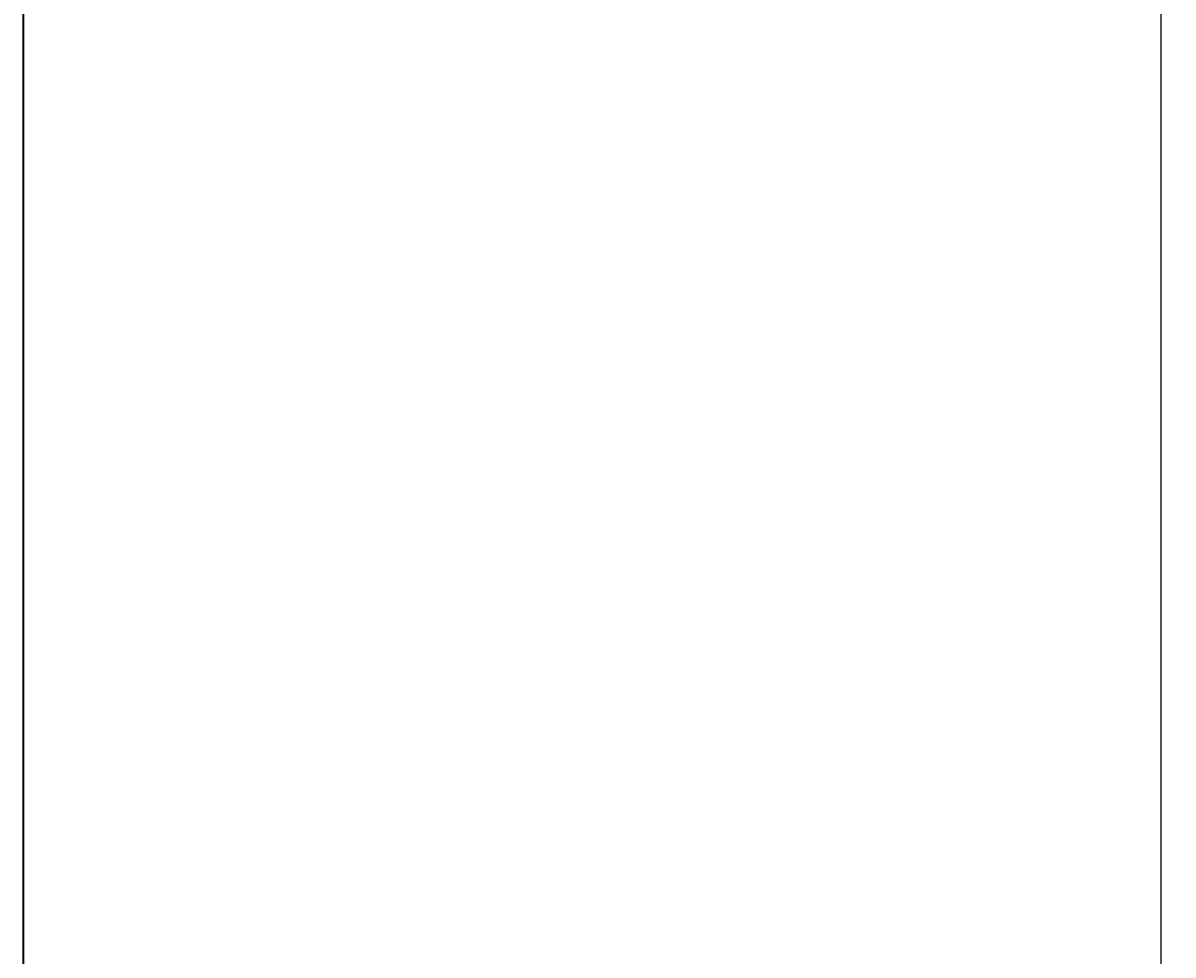
# Model space of a CAD drawing. Units: inches. Extents: x -128 to 854, y -395 to 398.
# Tile 34 of 61: x 314 to 352, y 64 to 95. Entities that reach past the tile are written whole.
import ezdxf

# ---------------------------------------------------------------- set-up
doc = ezdxf.new("R2010")
doc.units = ezdxf.units.IN
doc.header["$MEASUREMENT"] = 0
doc.layers.add('A-ANNO-DIMS', color=2, linetype='Continuous', lineweight=18)
doc.layers.add('A-WALL', color=4, linetype='Continuous', lineweight=35)
doc.styles.get("Standard").update_dxf_attribs({"font": 'arial.ttf'})
doc.dimstyles.get("Standard").update_dxf_attribs({"dimtxt": 0.18, "dimasz": 0.18, "dimexe": 0.18, "dimexo": 0.0625, "dimgap": 0.09, "dimtad": 0, "dimtih": 1, "dimtoh": 1, "dimdec": 1, "dimzin": 0, "dimdsep": 46, "dimlunit": 4, "dimtxsty": 'Standard', "dimcen": 0.09, "dimclrd": 1, "dimclre": 2, "dimclrt": 6, "dimadec": 0, "dimazin": 0, "dimtfac": 1, "dimtdec": 1, "dimtofl": 0, "dimtmove": 0, "dimatfit": 3, "dimfxl": 1, "dimtfill": 2, "dimtfillclr": 3, "dimtolj": 1, "dimtzin": 0, "dimarcsym": 0})

# ---------------------------------------------------------------- blocks, each defined once
blk = doc.blocks.new('*D98')
at = {"layer": 'A-ANNO-DIMS', "color": 2, "lineweight": -2, "transparency": 16777216}
for p, q in [((313.935, 348.741), (351.853, 348.741)), ((313.935, -89.259), (351.853, -89.259))]:
    blk.add_line(p, q, dxfattribs=at)
at = {"layer": 'A-ANNO-DIMS', "color": 1, "lineweight": -2, "transparency": 16777216}
for p, q in [((351.673, 348.561), (351.673, 129.923)), ((351.673, -89.079), (351.673, 129.559))]:
    blk.add_line(p, q, dxfattribs=at)
at = {"layer": 'A-ANNO-DIMS', "color": 1, "transparency": 16777216}
for points in [[(351.643, 348.561), (351.703, 348.561), (351.673, 348.741)], [(351.643, -89.079), (351.703, -89.079), (351.673, -89.259)]]:
    blk.add_solid(points, dxfattribs=at)
at = {"layer": 'Defpoints', "color": 0, "transparency": 16777216}
for p in [(313.873, 348.741), (351.673, 348.741), (313.873, -89.259)]:
    blk.add_point(p, dxfattribs=at)
at = {"layer": 'A-ANNO-DIMS', "color": 6, "transparency": 16777216, "insert": (351.673, 129.741), "char_height": 0.18, "attachment_point": 5, "bg_fill": 1, "box_fill_scale": 1.25, "bg_fill_color": 3, "bg_fill_transparency": 0}
blk.add_mtext('\\A1;36\'-6"', dxfattribs=at)

msp = doc.modelspace()

# ---------------------------------------------------------------- linework, layer by layer
at = {"layer": 'A-WALL'}
msp.add_line((313.873, 348.741), (313.873, -89.259), dxfattribs=at)

# ---------------------------------------------------------------- dimensions: what is measured, and where the dimension line sits
at = {"layer": 'A-ANNO-DIMS'}
dim = msp.add_linear_dim(base=(351.673, 348.741), p1=(313.873, -89.259), p2=(313.873, 348.741), angle=90, dimstyle='Standard', override={"dimdec": 1, "dimlfac": 1, "dimrnd": 0, "dimzin": 1, "dimdsep": 46, "dimlunit": 4, "dimfrac": 2}, dxfattribs=at)
dim.commit()
dim.dimension.update_dxf_attribs({"geometry": '*D98', "text_midpoint": (351.673, 129.741)})

doc.saveas('drawing.dxf')
